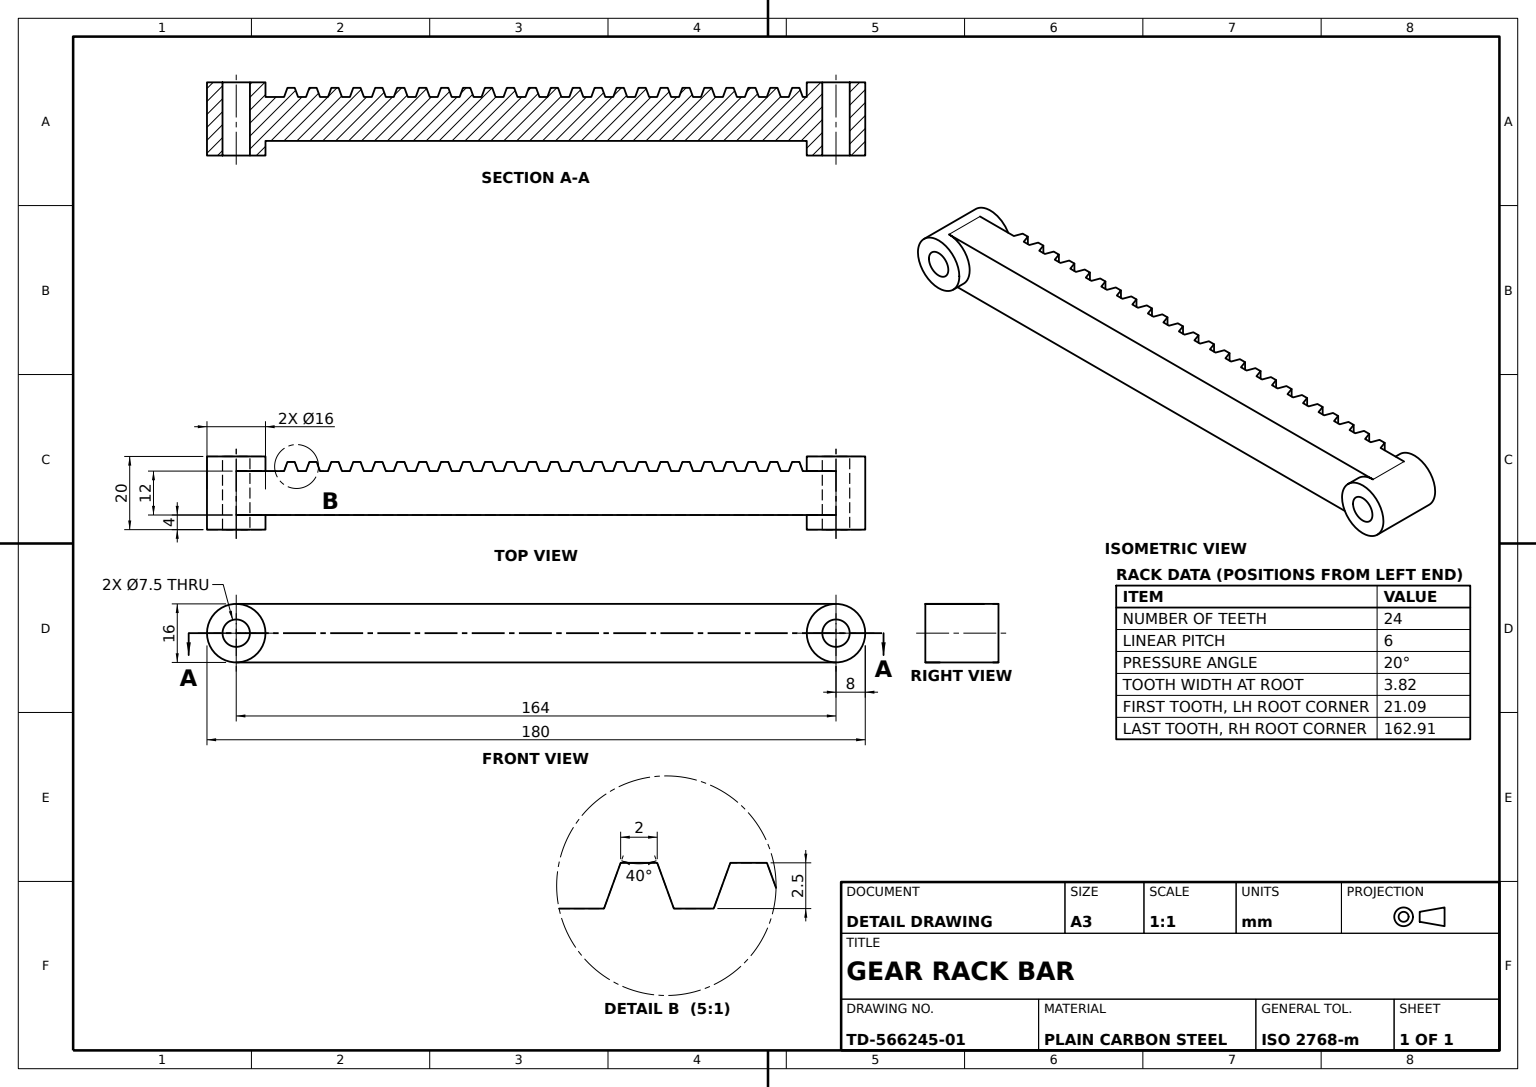
from build123d import *

# Parameters (mm, degrees)
EYE_BAR_PROFILE_SKETCH_R   = 8
EYE_BAR_PROFILE_SKETCH_R_2 = 3.75
BAR_WITH_EYE_ENDS_DEPTH    = 10
BAR_WITH_EYE_ENDS_2_DEPTH  = 10
RACK_BODY_DEPTH            = 6
RACK_TEETH_24X_DEPTH       = 8


with BuildPart() as part:
    # Eye Bar Profile Sketch → Bar With Eye Ends (new, symmetric)
    with BuildSketch(Plane(origin=(0, 0, 0), x_dir=(0, 0, -1), z_dir=(1, 0, 0))):
        Circle(EYE_BAR_PROFILE_SKETCH_R)
        Circle(EYE_BAR_PROFILE_SKETCH_R_2, mode=Mode.SUBTRACT)
    extrude(amount=BAR_WITH_EYE_ENDS_DEPTH, both=True)



with BuildPart() as body_2:
    # Eye Bar Profile Sketch → Bar With Eye Ends 2 (new, symmetric)
    with BuildSketch(Plane(origin=(0, 0, 0), x_dir=(0, 0, -1), z_dir=(1, 0, 0))):
        with Locations((-164, 0)):
            Circle(EYE_BAR_PROFILE_SKETCH_R)
        with Locations((-164, 0)):
            Circle(EYE_BAR_PROFILE_SKETCH_R_2, mode=Mode.SUBTRACT)
    extrude(amount=BAR_WITH_EYE_ENDS_2_DEPTH, both=True)


with BuildPart() as part_1:
    add(part.part)

    add(body_2.part)  # Rack Body merges body 2
    # Rack Body Sketch → Rack Body (add, symmetric)
    with BuildSketch(Plane(origin=(0, 0, 0), x_dir=(0, 0, -1), z_dir=(1, 0, 0))):
        with BuildLine():
            Line((-164, 8), (0, 8))
            ThreePointArc((0, 8), (-8, 0), (0, -8))
            Line((0, -8), (-164, -8))
            ThreePointArc((-164, -8), (-156, 0), (-164, 8))
        make_face()
    extrude(amount=RACK_BODY_DEPTH, both=True)

    # Rack Teeth Profile Sketch → Rack Teeth 24x (add, symmetric)
    with BuildSketch(Plane(origin=(0, 0, 0), x_dir=(1, 0, 0), z_dir=(0, 1, 0))):
        Polygon((-8.5, -10), (-8.5, -12), (-5.490653606, -13.095312512), (-5.490653606, -8.904687488), align=None)
        Polygon((-8.5, -16), (-5.490653606, -14.904687488), (-5.490653606, -19.095312512), (-8.5, -18), align=None)
        Polygon((-8.5, -22), (-5.490653606, -20.904687488), (-5.490653606, -25.095312512), (-8.5, -24), align=None)
        Polygon((-8.5, -28), (-5.490653606, -26.904687488), (-5.490653606, -31.095312512), (-8.5, -30), align=None)
        Polygon((-8.5, -34), (-5.490653606, -32.904687488), (-5.490653606, -37.095312512), (-8.5, -36), align=None)
        Polygon((-8.5, -40), (-5.490653606, -38.904687488), (-5.490653606, -43.095312512), (-8.5, -42), align=None)
        Polygon((-8.5, -46), (-5.490653606, -44.904687488), (-5.490653606, -49.095312512), (-8.5, -48), align=None)
        Polygon((-8.5, -52), (-5.490653606, -50.904687488), (-5.490653606, -55.095312512), (-8.5, -54), align=None)
        Polygon((-8.5, -58), (-5.490653606, -56.904687488), (-5.490653606, -61.095312512), (-8.5, -60), align=None)
        Polygon((-8.5, -64), (-5.490653606, -62.904687488), (-5.490653606, -67.095312512), (-8.5, -66), align=None)
        Polygon((-8.5, -70), (-5.490653606, -68.904687488), (-5.490653606, -73.095312512), (-8.5, -72), align=None)
        Polygon((-8.5, -76), (-5.490653606, -74.904687488), (-5.490653606, -79.095312512), (-8.5, -78), align=None)
        Polygon((-8.5, -82), (-5.490653606, -80.904687488), (-5.490653606, -85.095312512), (-8.5, -84), align=None)
        Polygon((-8.5, -88), (-5.490653606, -86.904687488), (-5.490653606, -91.095312512), (-8.5, -90), align=None)
        Polygon((-8.5, -94), (-5.490653606, -92.904687488), (-5.490653606, -97.095312512), (-8.5, -96), align=None)
        Polygon((-8.5, -100), (-5.490653606, -98.904687488), (-5.490653606, -103.095312512), (-8.5, -102), align=None)
        Polygon((-8.5, -106), (-5.490653606, -104.904687488), (-5.490653606, -109.095312512), (-8.5, -108), align=None)
        Polygon((-8.5, -112), (-5.490653606, -110.904687488), (-5.490653606, -115.095312512), (-8.5, -114), align=None)
        Polygon((-8.5, -118), (-5.490653606, -116.904687488), (-5.490653606, -121.095312512), (-8.5, -120), align=None)
        Polygon((-8.5, -124), (-5.490653606, -122.904687488), (-5.490653606, -127.095312512), (-8.5, -126), align=None)
        Polygon((-8.5, -130), (-5.490653606, -128.904687488), (-5.490653606, -133.095312512), (-8.5, -132), align=None)
        Polygon((-8.5, -136), (-5.490653606, -134.904687488), (-5.490653606, -139.095312512), (-8.5, -138), align=None)
        Polygon((-8.5, -142), (-5.490653606, -140.904687488), (-5.490653606, -145.095312512), (-8.5, -144), align=None)
        Polygon((-8.5, -148), (-5.490653606, -146.904687488), (-5.490653606, -151.095312512), (-8.5, -150), align=None)
    extrude(amount=RACK_TEETH_24X_DEPTH, both=True)


solid = part_1.part
